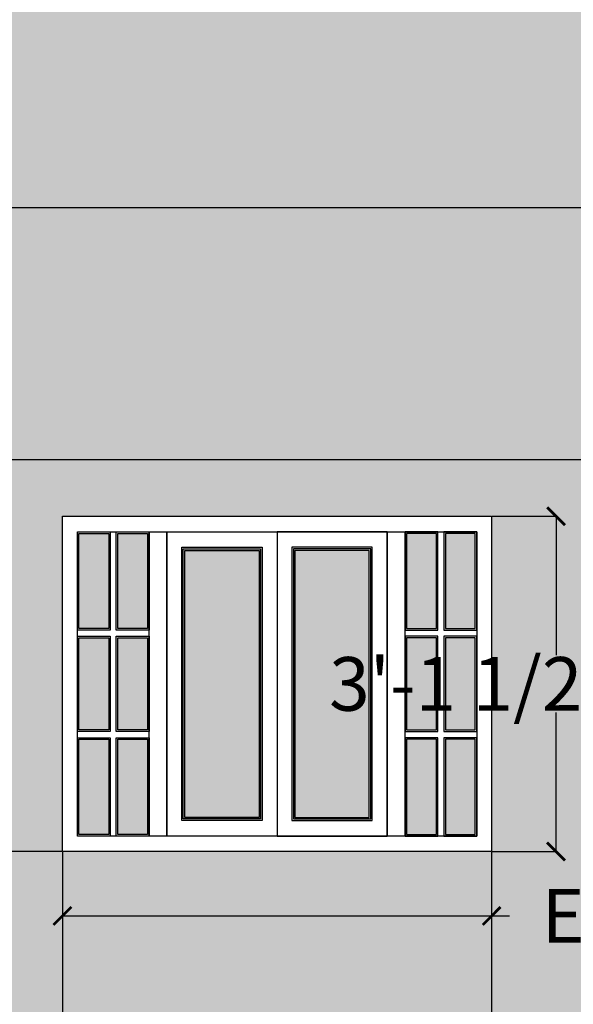
# Model space of a CAD drawing. Units: inches. Extents: x 528 to 2620, y -1066 to 798.
# Tile 37 of 41: x 2322 to 2384, y -1001 to -891. Entities that reach past the tile are written whole.
import ezdxf

# ---------------------------------------------------------------- set-up
doc = ezdxf.new("R2010")
doc.units = ezdxf.units.IN
doc.header["$MEASUREMENT"] = 0
for name, color, linetype, lineweight in [('A-ANNO-DIMS', 2, 'Continuous', 18), ('A-ELEV', 7, 'Continuous', 25), ('A-ELEV-PATT', 8, 'Continuous', 13)]:
    doc.layers.add(name, color=color, linetype=linetype, lineweight=lineweight)
doc.styles.get("Standard").update_dxf_attribs({"font": 'arial.ttf'})
doc.dimstyles.get("Standard").update_dxf_attribs({"dimtxt": 6, "dimasz": 2, "dimexe": 0.18, "dimexo": 0.0625, "dimgap": 0.09, "dimtad": 0, "dimtih": 1, "dimtoh": 1, "dimdec": 1, "dimzin": 0, "dimdsep": 46, "dimlunit": 3, "dimtxsty": 'Standard', "dimblk": 'ARCHTICK', "dimcen": 0.09, "dimadec": 0, "dimazin": 0, "dimtfac": 1, "dimtdec": 1, "dimtofl": 0, "dimtmove": 0, "dimatfit": 3, "dimfxl": 1, "dimtolj": 1, "dimtzin": 0, "dimarcsym": 0})

# ---------------------------------------------------------------- blocks, each defined once
blk = doc.blocks.new('ww')
at = {"color": 0, "linetype": 'ByBlock'}
for p, q in [((30.67, -16.13), (126.65, -16.13)), ((30.67, -91.08), (30.67, -16.13)), ((126.65, -16.13), (126.65, -91.08)), ((34.01, -19.6), (123.32, -19.6)), ((34.01, -87.61), (34.01, -19.6)), ((34.01, -19.6), (49.87, -19.6)), ((34.01, -87.61), (34.01, -19.6)), ((50.03, -87.61), (50.03, -19.6)), ((54.03, -19.6), (54.03, -87.61)), ((103.29, -19.6), (103.29, -87.61)), ((107.29, -87.61), (107.29, -19.6)), ((123.32, -19.6), (123.32, -87.61)), ((123.32, -87.61), (34.01, -87.61)), ((126.65, -91.08), (30.67, -91.08))]:
    blk.add_line(p, q, dxfattribs=at)
at = {"color": 0, "linetype": 'ByBlock', "ltscale": 25}
for p, q in [((34.01, -41.58), (34.01, -19.6)), ((34.01, -19.6), (41.35, -19.6)), ((41.35, -19.6), (41.35, -41.58)), ((42.69, -41.58), (42.69, -19.6)), ((42.69, -19.6), (50.03, -19.6)), ((50.03, -19.6), (50.03, -41.58)), ((54.03, -87.61), (54.03, -19.6)), ((54.03, -19.6), (78.66, -19.6)), ((103.29, -19.6), (78.66, -19.6)), ((78.66, -19.6), (78.66, -87.61)), ((78.66, -19.6), (78.66, -87.61)), ((103.29, -87.61), (103.29, -19.6)), ((107.29, -19.6), (107.29, -41.58)), ((114.63, -19.6), (107.29, -19.6)), ((114.63, -41.58), (114.63, -19.6)), ((115.97, -19.6), (115.97, -41.58)), ((123.32, -19.6), (115.97, -19.6)), ((123.32, -41.58), (123.32, -19.6)), ((34.34, -41.23), (34.34, -19.95)), ((34.34, -19.95), (41.02, -19.95)), ((41.02, -19.95), (41.02, -41.23)), ((43.02, -41.23), (43.02, -19.95)), ((43.02, -19.95), (49.7, -19.95)), ((49.7, -19.95), (49.7, -41.23)), ((107.62, -19.95), (107.62, -41.23)), ((114.3, -19.95), (107.62, -19.95)), ((114.3, -41.23), (114.3, -19.95)), ((116.3, -19.95), (116.3, -41.23)), ((122.98, -19.95), (116.3, -19.95)), ((122.98, -41.23), (122.98, -19.95)), ((57.37, -84.14), (57.37, -23.07)), ((57.37, -23.07), (75.33, -23.07)), ((57.7, -83.8), (57.7, -23.42)), ((57.7, -23.42), (74.99, -23.42)), ((58.03, -83.45), (58.03, -23.77)), ((58.03, -23.77), (74.66, -23.77)), ((74.66, -23.77), (74.66, -83.45)), ((74.99, -23.42), (74.99, -83.8)), ((75.33, -23.07), (75.33, -84.14)), ((99.96, -23.07), (81.99, -23.07)), ((81.99, -23.07), (81.99, -84.14)), ((99.62, -23.42), (82.33, -23.42)), ((82.33, -23.42), (82.33, -83.8)), ((99.29, -23.77), (82.66, -23.77)), ((82.66, -23.77), (82.66, -83.45)), ((99.29, -83.45), (99.29, -23.77)), ((99.62, -83.8), (99.62, -23.42)), ((99.96, -84.14), (99.96, -23.07)), ((41.35, -41.58), (34.01, -41.58)), ((41.02, -41.23), (34.34, -41.23)), ((50.03, -41.58), (42.69, -41.58)), ((49.7, -41.23), (43.02, -41.23)), ((107.29, -41.58), (114.63, -41.58)), ((107.62, -41.23), (114.3, -41.23)), ((115.97, -41.58), (123.32, -41.58)), ((116.3, -41.23), (122.98, -41.23)), ((34.01, -64.25), (34.01, -42.97)), ((34.01, -42.97), (41.35, -42.97)), ((34.34, -63.9), (34.34, -43.31)), ((34.34, -43.31), (41.02, -43.31)), ((41.02, -43.31), (41.02, -63.9)), ((41.35, -42.97), (41.35, -64.25)), ((42.69, -64.25), (42.69, -42.97)), ((42.69, -42.97), (50.03, -42.97)), ((43.02, -63.9), (43.02, -43.31)), ((43.02, -43.31), (49.7, -43.31)), ((49.7, -43.31), (49.7, -63.9)), ((50.03, -42.97), (50.03, -64.25)), ((107.29, -42.97), (107.29, -64.25)), ((114.63, -42.97), (107.29, -42.97)), ((107.62, -43.31), (107.62, -63.9)), ((114.3, -43.31), (107.62, -43.31)), ((114.3, -63.9), (114.3, -43.31)), ((114.63, -64.25), (114.63, -42.97)), ((115.97, -42.97), (115.97, -64.25)), ((123.32, -42.97), (115.97, -42.97)), ((116.3, -43.31), (116.3, -63.9)), ((122.98, -43.31), (116.3, -43.31)), ((122.98, -63.9), (122.98, -43.31)), ((123.32, -64.25), (123.32, -42.97)), ((41.35, -64.25), (34.01, -64.25)), ((34.01, -87.61), (34.01, -65.64)), ((34.01, -65.64), (41.35, -65.64)), ((41.02, -63.9), (34.34, -63.9)), ((34.34, -87.27), (34.34, -65.98)), ((34.34, -65.98), (41.02, -65.98)), ((41.02, -65.98), (41.02, -87.27)), ((41.35, -65.64), (41.35, -87.61)), ((50.03, -64.25), (42.69, -64.25)), ((42.69, -87.61), (42.69, -65.64)), ((42.69, -65.64), (50.03, -65.64)), ((49.7, -63.9), (43.02, -63.9)), ((43.02, -87.27), (43.02, -65.98)), ((43.02, -65.98), (49.7, -65.98)), ((49.7, -65.98), (49.7, -87.27)), ((50.03, -65.64), (50.03, -87.61)), ((107.29, -64.25), (114.63, -64.25)), ((107.29, -65.64), (107.29, -87.61)), ((114.63, -65.64), (107.29, -65.64)), ((107.62, -63.9), (114.3, -63.9)), ((107.62, -65.98), (107.62, -87.27)), ((114.3, -65.98), (107.62, -65.98)), ((114.3, -87.27), (114.3, -65.98)), ((114.63, -87.61), (114.63, -65.64)), ((115.97, -64.25), (123.32, -64.25)), ((115.97, -65.64), (115.97, -87.61)), ((123.32, -65.64), (115.97, -65.64)), ((116.3, -63.9), (122.98, -63.9)), ((116.3, -65.98), (116.3, -87.27)), ((122.98, -65.98), (116.3, -65.98)), ((122.98, -87.27), (122.98, -65.98)), ((123.32, -87.61), (123.32, -65.64)), ((74.66, -83.45), (58.03, -83.45)), ((82.66, -83.45), (99.29, -83.45)), ((75.33, -84.14), (57.37, -84.14)), ((74.99, -83.8), (57.7, -83.8)), ((81.99, -84.14), (99.96, -84.14)), ((82.33, -83.8), (99.62, -83.8)), ((41.35, -87.61), (34.01, -87.61)), ((41.02, -87.27), (34.34, -87.27)), ((50.03, -87.61), (42.69, -87.61)), ((49.7, -87.27), (43.02, -87.27)), ((78.66, -87.61), (54.03, -87.61)), ((78.66, -87.61), (103.29, -87.61)), ((107.29, -87.61), (114.63, -87.61)), ((107.62, -87.27), (114.3, -87.27)), ((115.97, -87.61), (123.32, -87.61)), ((116.3, -87.27), (122.98, -87.27))]:
    blk.add_line(p, q, dxfattribs=at)
blk = doc.blocks.new('_ArchTick')
at = {"color": 0, "linetype": 'ByBlock', "const_width": 0.15}
blk.add_lwpolyline([(-0.5, -0.5), (0.5, 0.5)], dxfattribs=at)
blk = doc.blocks.new('*D54')
at = {"layer": 'A-ANNO-DIMS', "color": 0, "lineweight": -2, "transparency": 16777216}
for p, q in [((2327.05, -984.21), (2327.05, -991.53)), ((2375.05, -984.21), (2375.05, -991.53)), ((2327.05, -991.35), (2375.05, -991.35)), ((2375.05, -991.35), (2377.05, -991.35))]:
    blk.add_line(p, q, dxfattribs=at)
at = {"layer": 'Defpoints', "color": 0, "transparency": 16777216}
for p in [(2327.05, -984.15), (2375.05, -984.15), (2375.05, -991.35)]:
    blk.add_point(p, dxfattribs=at)
at = {"layer": 'A-ANNO-DIMS', "color": 0, "lineweight": -2, "transparency": 16777216, "xscale": 2, "yscale": 2, "zscale": 2, "rotation": 180}
blk.add_blockref('_ArchTick', (2327.05, -991.35), dxfattribs=at)
at = {"layer": 'A-ANNO-DIMS', "color": 0, "lineweight": -2, "transparency": 16777216, "xscale": 2, "yscale": 2, "zscale": 2}
blk.add_blockref('_ArchTick', (2375.05, -991.35), dxfattribs=at)
at = {"layer": 'A-ANNO-DIMS', "color": 0, "transparency": 16777216, "insert": (2439.5, -991.35), "char_height": 6, "attachment_point": 5}
blk.add_mtext('\\A1;ELEVATION WINDOW 4\'-0" TYP.', dxfattribs=at)
blk = doc.blocks.new('*D55')
at = {"layer": 'A-ANNO-DIMS', "color": 0, "lineweight": -2, "transparency": 16777216}
for p, q in [((2375.11, -946.66), (2382.43, -946.66)), ((2382.25, -946.66), (2382.25, -962.21)), ((2382.25, -984.15), (2382.25, -968.6)), ((2375.11, -984.15), (2382.43, -984.15))]:
    blk.add_line(p, q, dxfattribs=at)
at = {"layer": 'Defpoints', "color": 0, "transparency": 16777216}
for p in [(2375.05, -946.66), (2382.25, -946.66), (2375.05, -984.15)]:
    blk.add_point(p, dxfattribs=at)
at = {"layer": 'A-ANNO-DIMS', "color": 0, "lineweight": -2, "transparency": 16777216, "xscale": 2, "yscale": 2, "zscale": 2}
for p, rotation in [((2382.25, -946.66), 90), ((2382.25, -984.15), 270)]:
    blk.add_blockref('_ArchTick', p, dxfattribs=dict(at, rotation=rotation))
at = {"layer": 'A-ANNO-DIMS', "color": 0, "transparency": 16777216, "insert": (2382.25, -965.41), "char_height": 6, "attachment_point": 5}
blk.add_mtext('\\A1;3\'-1 1/2" TYP.', dxfattribs=at)
blk = doc.blocks.new('*D71')
at = {"layer": 'A-ANNO-DIMS', "color": 0, "lineweight": -2, "transparency": 16777216}
for p, q in [((2326.98, -984.15), (2243.87, -984.15)), ((2244.05, -984.15), (2244.05, -998.99)), ((2244.05, -1020.15), (2244.05, -1005.3)), ((2298.48, -1020.15), (2243.87, -1020.15))]:
    blk.add_line(p, q, dxfattribs=at)
at = {"layer": 'Defpoints', "color": 0, "transparency": 16777216}
for p in [(2244.05, -984.15), (2327.05, -984.15), (2298.55, -1020.15)]:
    blk.add_point(p, dxfattribs=at)
at = {"layer": 'A-ANNO-DIMS', "color": 0, "lineweight": -2, "transparency": 16777216, "xscale": 2, "yscale": 2, "zscale": 2}
for p, rotation in [((2244.05, -984.15), 90), ((2244.05, -1020.15), 270)]:
    blk.add_blockref('_ArchTick', p, dxfattribs=dict(at, rotation=rotation))
at = {"layer": 'A-ANNO-DIMS', "color": 0, "transparency": 16777216, "insert": (2244.05, -1002.15), "char_height": 6, "attachment_point": 5}
blk.add_mtext('\\A1;3\'-0"', dxfattribs=at)
blk = doc.blocks.new('*D72')
at = {"layer": 'A-ANNO-DIMS', "color": 0, "lineweight": -2, "transparency": 16777216}
for p, q in [((2394.48, -940.36), (2243.87, -940.36)), ((2244.05, -940.36), (2244.05, -959.1)), ((2244.05, -984.15), (2244.05, -965.41)), ((2326.98, -984.15), (2243.87, -984.15))]:
    blk.add_line(p, q, dxfattribs=at)
at = {"layer": 'Defpoints', "color": 0, "transparency": 16777216}
for p in [(2244.05, -940.36), (2394.55, -940.36), (2327.05, -984.15)]:
    blk.add_point(p, dxfattribs=at)
at = {"layer": 'A-ANNO-DIMS', "color": 0, "lineweight": -2, "transparency": 16777216, "xscale": 2, "yscale": 2, "zscale": 2}
for p, rotation in [((2244.05, -940.36), 90), ((2244.05, -984.15), 270)]:
    blk.add_blockref('_ArchTick', p, dxfattribs=dict(at, rotation=rotation))
at = {"layer": 'A-ANNO-DIMS', "color": 0, "transparency": 16777216, "insert": (2244.05, -962.26), "char_height": 6, "attachment_point": 5}
blk.add_mtext('\\A1;3\'-8"', dxfattribs=at)
blk = doc.blocks.new('*D73')
at = {"layer": 'A-ANNO-DIMS', "color": 0, "lineweight": -2, "transparency": 16777216}
for p, q in [((2265.98, -912.15), (2243.87, -912.15)), ((2244.05, -912.15), (2244.05, -923.15)), ((2244.05, -940.36), (2244.05, -929.36)), ((2394.48, -940.36), (2243.87, -940.36))]:
    blk.add_line(p, q, dxfattribs=at)
at = {"layer": 'Defpoints', "color": 0, "transparency": 16777216}
for p in [(2244.05, -912.15), (2266.05, -912.15), (2394.55, -940.36)]:
    blk.add_point(p, dxfattribs=at)
at = {"layer": 'A-ANNO-DIMS', "color": 0, "lineweight": -2, "transparency": 16777216, "xscale": 2, "yscale": 2, "zscale": 2}
for p, rotation in [((2244.05, -912.15), 90), ((2244.05, -940.36), 270)]:
    blk.add_blockref('_ArchTick', p, dxfattribs=dict(at, rotation=rotation))
at = {"layer": 'A-ANNO-DIMS', "color": 0, "transparency": 16777216, "insert": (2244.05, -926.26), "char_height": 6, "attachment_point": 5}
blk.add_mtext('\\A1;2\'-4"', dxfattribs=at)
blk = doc.blocks.new('*D81')
at = {"layer": 'A-ANNO-DIMS', "color": 0, "lineweight": -2, "transparency": 16777216}
for p, q in [((2327.05, -984.21), (2327.05, -1042.33)), ((2298.55, -1020.21), (2298.55, -1042.33)), ((2298.55, -1042.15), (2327.05, -1042.15)), ((2327.05, -1042.15), (2329.05, -1042.15))]:
    blk.add_line(p, q, dxfattribs=at)
at = {"layer": 'Defpoints', "color": 0, "transparency": 16777216}
for p in [(2327.05, -984.15), (2298.55, -1020.15), (2327.05, -1042.15)]:
    blk.add_point(p, dxfattribs=at)
at = {"layer": 'A-ANNO-DIMS', "color": 0, "lineweight": -2, "transparency": 16777216, "xscale": 2, "yscale": 2, "zscale": 2, "rotation": 180}
blk.add_blockref('_ArchTick', (2298.55, -1042.15), dxfattribs=at)
at = {"layer": 'A-ANNO-DIMS', "color": 0, "lineweight": -2, "transparency": 16777216, "xscale": 2, "yscale": 2, "zscale": 2}
blk.add_blockref('_ArchTick', (2327.05, -1042.15), dxfattribs=at)
at = {"layer": 'A-ANNO-DIMS', "color": 0, "transparency": 16777216, "insert": (2344.15, -1042.15), "char_height": 6, "attachment_point": 5}
blk.add_mtext('\\A1;2\'-4 1/2"', dxfattribs=at)
blk = doc.blocks.new('*D82')
at = {"layer": 'A-ANNO-DIMS', "color": 0, "lineweight": -2, "transparency": 16777216}
for p, q in [((2327.05, -984.21), (2327.05, -1042.33)), ((2375.05, -984.21), (2375.05, -1042.33)), ((2327.05, -1042.15), (2342.86, -1042.15)), ((2375.05, -1042.15), (2359.23, -1042.15))]:
    blk.add_line(p, q, dxfattribs=at)
at = {"layer": 'Defpoints', "color": 0, "transparency": 16777216}
for p in [(2327.05, -984.15), (2375.05, -984.15), (2375.05, -1042.15)]:
    blk.add_point(p, dxfattribs=at)
at = {"layer": 'A-ANNO-DIMS', "color": 0, "lineweight": -2, "transparency": 16777216, "xscale": 2, "yscale": 2, "zscale": 2, "rotation": 180}
blk.add_blockref('_ArchTick', (2327.05, -1042.15), dxfattribs=at)
at = {"layer": 'A-ANNO-DIMS', "color": 0, "lineweight": -2, "transparency": 16777216, "xscale": 2, "yscale": 2, "zscale": 2}
blk.add_blockref('_ArchTick', (2375.05, -1042.15), dxfattribs=at)
at = {"layer": 'A-ANNO-DIMS', "color": 0, "transparency": 16777216, "insert": (2351.05, -1042.15), "char_height": 6, "attachment_point": 5}
blk.add_mtext('\\A1;4\'-0"', dxfattribs=at)
blk = doc.blocks.new('*D83')
at = {"layer": 'A-ANNO-DIMS', "color": 0, "lineweight": -2, "transparency": 16777216}
for p, q in [((2375.05, -984.21), (2375.05, -1042.33)), ((2394.55, -1020.21), (2394.55, -1042.33)), ((2375.05, -1042.15), (2394.55, -1042.15)), ((2394.55, -1042.15), (2396.55, -1042.15))]:
    blk.add_line(p, q, dxfattribs=at)
at = {"layer": 'Defpoints', "color": 0, "transparency": 16777216}
for p in [(2375.05, -984.15), (2394.55, -1020.15), (2394.55, -1042.15)]:
    blk.add_point(p, dxfattribs=at)
at = {"layer": 'A-ANNO-DIMS', "color": 0, "lineweight": -2, "transparency": 16777216, "xscale": 2, "yscale": 2, "zscale": 2, "rotation": 180}
blk.add_blockref('_ArchTick', (2375.05, -1042.15), dxfattribs=at)
at = {"layer": 'A-ANNO-DIMS', "color": 0, "lineweight": -2, "transparency": 16777216, "xscale": 2, "yscale": 2, "zscale": 2}
blk.add_blockref('_ArchTick', (2394.55, -1042.15), dxfattribs=at)
at = {"layer": 'A-ANNO-DIMS', "color": 0, "transparency": 16777216, "insert": (2411.32, -1042.15), "char_height": 6, "attachment_point": 5}
blk.add_mtext('\\A1;1\'-7 1/2"', dxfattribs=at)

msp = doc.modelspace()

# ---------------------------------------------------------------- hatches: boundary and pattern name
at = {"layer": 'A-ELEV-PATT', "transparency": 33554687}
h = msp.add_hatch(color=256, dxfattribs=at)
h.dxf.hatch_style = 1
h.paths.add_polyline_path([(2448.55, -756.15), (2270.55, -756.15), (2270.55, -780.15), (2436.55, -780.15), (2436.55, -888.15), (2266.05, -888.15), (2266.05, -912.15), (2448.55, -912.15)])
h = msp.add_hatch(color=256, dxfattribs=at)
h.dxf.hatch_style = 1
h.paths.add_polyline_path([(2586.55, -912.15), (2448.55, -912.15), (2448.55, -940.66), (2547.55, -940.66), (2547.55, -990.15), (2448.55, -990.15), (2448.55, -1020.15), (2586.55, -1020.15)])
h.paths.add_polyline_path([(2481.55, -789.84), (2562.55, -789.84), (2562.55, -761.55), (2448.55, -761.55), (2448.55, -900.15), (2562.55, -900.15), (2562.55, -876.97), (2481.55, -876.97), (2481.55, -833.41)])
h.paths.add_polyline_path([(2412.55, -780.15), (2298.55, -780.15), (2298.55, -852.15), (2322.55, -852.15), (2322.55, -814.66), (2370.55, -814.66), (2370.55, -852.15), (2412.55, -852.15)])
h.paths.add_polyline_path([(2394.55, -940.36), (2442.55, -940.36), (2442.55, -1020.15), (2448.55, -1020.15), (2448.55, -990.15), (2448.55, -912.15), (2310.55, -912.15), (2310.55, -1020.15), (2394.55, -1020.15)])
h.paths.add_polyline_path([(2327.05, -984.15), (2327.05, -946.66), (2375.05, -946.66), (2375.05, -984.15)], flags=16)
h.paths.add_polyline_path([(2328.71, -982.41), (2328.71, -948.4), (2336.65, -948.4), (2336.73, -948.4), (2373.38, -948.4), (2373.38, -982.41), (2369.7, -982.41)], flags=0)
h.paths.add_polyline_path([(2338.73, -982.41), (2338.73, -948.4), (2351.05, -948.4), (2363.36, -948.4), (2363.36, -982.41), (2351.05, -982.41)], flags=0)
h.paths.add_polyline_path([(2340.4, -980.68), (2340.4, -950.13), (2349.38, -950.13), (2349.38, -980.68)], flags=0)
h.paths.add_polyline_path([(2340.73, -980.33), (2340.73, -950.48), (2349.05, -950.48), (2349.05, -980.33)], flags=0)
h.paths.add_polyline_path([(2352.71, -980.68), (2352.71, -950.13), (2361.7, -950.13), (2361.7, -980.68)], flags=0)
h.paths.add_polyline_path([(2353.05, -980.33), (2353.05, -950.48), (2361.36, -950.48), (2361.36, -980.33)], flags=0)
h.paths.add_polyline_path([(2336.73, -982.41), (2333.05, -982.41), (2333.05, -971.42), (2336.73, -971.42), (2336.73, -970.73), (2333.05, -970.73), (2333.05, -960.08), (2336.73, -960.08), (2336.73, -959.39), (2333.05, -959.39), (2333.05, -948.57), (2336.73, -948.57)], flags=0)
h.paths.add_polyline_path([(2333.22, -982.24), (2333.22, -971.6), (2336.73, -971.6), (2336.73, -982.24)], flags=0)
h.paths.add_polyline_path([(2332.39, -982.41), (2328.71, -982.41), (2328.71, -948.4), (2332.39, -948.4), (2332.39, -959.39), (2328.71, -959.39), (2328.71, -960.08), (2332.39, -960.08), (2332.39, -970.73), (2328.71, -970.73), (2328.71, -971.42), (2332.39, -971.42)], flags=0)
h.paths.add_polyline_path([(2332.22, -982.24), (2328.71, -982.24), (2328.71, -971.6), (2332.22, -971.6)], flags=0)
h.paths.add_polyline_path([(2365.36, -982.41), (2365.36, -948.4), (2369.04, -948.4), (2369.04, -959.39), (2365.36, -959.39), (2365.36, -960.08), (2369.04, -960.08), (2369.04, -970.73), (2365.36, -970.73), (2365.36, -971.42), (2369.04, -971.42), (2369.04, -982.41)], flags=0)
h.paths.add_polyline_path([(2369.7, -971.42), (2373.38, -971.42), (2373.38, -982.24), (2369.7, -982.24)], flags=0)
h.paths.add_polyline_path([(2333.22, -970.55), (2333.22, -960.26), (2336.73, -960.26), (2336.73, -970.55)], flags=0)
h.paths.add_polyline_path([(2332.22, -970.55), (2328.71, -970.55), (2328.71, -960.26), (2332.22, -960.26)], flags=0)
h.paths.add_polyline_path([(2369.7, -970.73), (2369.7, -960.08), (2373.38, -960.08), (2373.38, -970.73)], flags=0)
h.paths.add_polyline_path([(2336.56, -959.22), (2336.56, -948.57), (2336.73, -948.4), (2336.73, -959.22)], flags=0)
h.paths.add_polyline_path([(2332.22, -959.22), (2328.71, -959.22), (2328.71, -948.57), (2332.22, -948.57)], flags=0)
h.paths.add_polyline_path([(2369.7, -959.39), (2369.7, -948.4), (2373.38, -948.4), (2373.38, -959.39)], flags=0)
h = msp.add_hatch(color=256, dxfattribs=at)
h.dxf.hatch_style = 1
h.paths.add_polyline_path([(2527.86, -818.48), (2519.55, -818.48), (2519.55, -848.33), (2527.86, -848.33)])
h.paths.add_polyline_path([(2515.55, -818.48), (2507.23, -818.48), (2507.23, -848.33), (2515.55, -848.33)])
h.paths.add_polyline_path([(2498.72, -816.57), (2495.38, -816.57), (2495.38, -827.22), (2498.72, -827.22)])
h.paths.add_polyline_path([(2503.06, -816.57), (2499.72, -816.57), (2499.72, -827.22), (2503.06, -827.22)])
h.paths.add_polyline_path([(2498.72, -828.26), (2495.38, -828.26), (2495.38, -838.55), (2498.72, -838.55)])
h.paths.add_polyline_path([(2503.06, -828.26), (2499.72, -828.26), (2499.72, -838.55), (2503.06, -838.55)])
h.paths.add_polyline_path([(2498.72, -839.6), (2495.38, -839.6), (2495.38, -850.24), (2498.72, -850.24)])
h.paths.add_polyline_path([(2503.06, -839.6), (2499.72, -839.6), (2499.72, -850.24), (2503.06, -850.24)])
h.paths.add_polyline_path([(2535.37, -839.6), (2532.03, -839.6), (2532.03, -850.24), (2535.37, -850.24)])
h.paths.add_polyline_path([(2539.71, -839.6), (2536.37, -839.6), (2536.37, -850.24), (2539.71, -850.24)])
h.paths.add_polyline_path([(2535.37, -828.26), (2532.03, -828.26), (2532.03, -838.55), (2535.37, -838.55)])
h.paths.add_polyline_path([(2539.71, -828.26), (2536.37, -828.26), (2536.37, -838.55), (2539.71, -838.55)])
h.paths.add_polyline_path([(2535.37, -816.57), (2532.03, -816.57), (2532.03, -827.22), (2535.37, -827.22)])
h.paths.add_polyline_path([(2356.86, -818.48), (2348.55, -818.48), (2348.55, -848.33), (2356.86, -848.33)])
h.paths.add_polyline_path([(2344.55, -818.48), (2336.23, -818.48), (2336.23, -848.33), (2344.55, -848.33)])
h.paths.add_polyline_path([(2327.72, -816.57), (2324.38, -816.57), (2324.38, -827.22), (2327.72, -827.22)])
h.paths.add_polyline_path([(2332.06, -816.57), (2328.72, -816.57), (2328.72, -827.22), (2332.06, -827.22)])
h.paths.add_polyline_path([(2327.72, -828.26), (2324.38, -828.26), (2324.38, -838.55), (2327.72, -838.55)])
h.paths.add_polyline_path([(2332.06, -828.26), (2328.72, -828.26), (2328.72, -838.55), (2332.06, -838.55)])
h.paths.add_polyline_path([(2327.72, -839.6), (2324.38, -839.6), (2324.38, -850.24), (2327.72, -850.24)])
h.paths.add_polyline_path([(2332.06, -839.6), (2328.72, -839.6), (2328.72, -850.24), (2332.06, -850.24)])
h.paths.add_polyline_path([(2368.71, -839.6), (2365.37, -839.6), (2365.37, -850.24), (2368.71, -850.24)])
h.paths.add_polyline_path([(2364.37, -839.6), (2361.03, -839.6), (2361.03, -850.24), (2364.37, -850.24)])
h.paths.add_polyline_path([(2364.37, -828.26), (2361.03, -828.26), (2361.03, -838.55), (2364.37, -838.55)])
h.paths.add_polyline_path([(2368.71, -828.26), (2365.37, -828.26), (2365.37, -838.55), (2368.71, -838.55)])
h.paths.add_polyline_path([(2364.37, -816.57), (2361.03, -816.57), (2361.03, -827.22), (2364.37, -827.22)])
h.paths.add_polyline_path([(2368.71, -816.57), (2365.37, -816.57), (2365.37, -827.22), (2368.71, -827.22)])
h.paths.add_polyline_path([(2361.36, -950.48), (2353.05, -950.48), (2353.05, -980.33), (2361.36, -980.33)])
h.paths.add_polyline_path([(2349.05, -950.48), (2340.73, -950.48), (2340.73, -980.33), (2349.05, -980.33)])
h.paths.add_polyline_path([(2336.56, -971.6), (2333.22, -971.6), (2333.22, -982.24), (2336.56, -982.24)])
h.paths.add_polyline_path([(2332.22, -971.6), (2328.88, -971.6), (2328.88, -982.24), (2332.22, -982.24)])
h.paths.add_polyline_path([(2336.56, -960.26), (2333.22, -960.26), (2333.22, -970.55), (2336.56, -970.55)])
h.paths.add_polyline_path([(2332.22, -960.26), (2328.88, -960.26), (2328.88, -970.55), (2332.22, -970.55)])
h.paths.add_polyline_path([(2332.22, -948.57), (2328.88, -948.57), (2328.88, -959.22), (2332.22, -959.22)])
h.paths.add_polyline_path([(2336.56, -948.57), (2333.22, -948.57), (2333.22, -959.22), (2336.56, -959.22)])
h.paths.add_polyline_path([(2368.87, -971.6), (2365.53, -971.6), (2365.53, -982.24), (2368.87, -982.24)])
h.paths.add_polyline_path([(2373.21, -971.6), (2369.87, -971.6), (2369.87, -982.24), (2373.21, -982.24)])
h.paths.add_polyline_path([(2373.21, -960.26), (2369.87, -960.26), (2369.87, -970.55), (2373.21, -970.55)])
h.paths.add_polyline_path([(2368.87, -960.26), (2365.53, -960.26), (2365.53, -970.55), (2368.87, -970.55)])
h.paths.add_polyline_path([(2368.87, -948.57), (2365.53, -948.57), (2365.53, -959.22), (2368.87, -959.22)])
h.paths.add_polyline_path([(2373.21, -948.57), (2369.87, -948.57), (2369.87, -959.22), (2373.21, -959.22)])
h.paths.add_polyline_path([(2527.86, -950.48), (2519.55, -950.48), (2519.55, -980.33), (2527.86, -980.33)])
h.paths.add_polyline_path([(2515.55, -950.48), (2507.23, -950.48), (2507.23, -980.33), (2515.55, -980.33)])
h.paths.add_polyline_path([(2539.71, -971.6), (2536.37, -971.6), (2536.37, -982.24), (2539.71, -982.24)])
h.paths.add_polyline_path([(2535.37, -971.6), (2532.03, -971.6), (2532.03, -982.24), (2535.37, -982.24)])
h.paths.add_polyline_path([(2535.37, -960.26), (2532.03, -960.26), (2532.03, -970.55), (2535.37, -970.55)])
h.paths.add_polyline_path([(2539.71, -960.26), (2536.37, -960.26), (2536.37, -970.55), (2539.71, -970.55)])
h.paths.add_polyline_path([(2535.37, -948.57), (2532.03, -948.57), (2532.03, -959.22), (2535.37, -959.22)])
h.paths.add_polyline_path([(2539.71, -948.57), (2536.37, -948.57), (2536.37, -959.22), (2539.71, -959.22)])
h.paths.add_polyline_path([(2498.72, -971.6), (2495.38, -971.6), (2495.38, -982.24), (2498.72, -982.24)])
h.paths.add_polyline_path([(2503.06, -971.6), (2499.72, -971.6), (2499.72, -982.24), (2503.06, -982.24)])
h.paths.add_polyline_path([(2498.72, -960.26), (2495.38, -960.26), (2495.38, -970.55), (2498.72, -970.55)])
h.paths.add_polyline_path([(2503.06, -960.26), (2499.72, -960.26), (2499.72, -970.55), (2503.06, -970.55)])
h.paths.add_polyline_path([(2498.72, -948.57), (2495.38, -948.57), (2495.38, -959.22), (2498.72, -959.22)])
h.paths.add_polyline_path([(2503.06, -948.57), (2499.72, -948.57), (2499.72, -959.22), (2503.06, -959.22)])

# ---------------------------------------------------------------- linework, layer by layer
at = {"layer": 'A-ELEV'}
msp.add_line((2266.05, -912.15), (2448.55, -912.15), dxfattribs=at)

# ---------------------------------------------------------------- block references
at = {"layer": 'A-ELEV', "xscale": 0.5001250312578946, "yscale": 0.5001250312578946, "zscale": 0.5001250312578946}
msp.add_blockref('ww', (2311.71, -938.6), dxfattribs=at)

# ---------------------------------------------------------------- dimensions: what is measured, and where the dimension line sits
at = {"layer": 'A-ANNO-DIMS'}
for base, p1, p2, picture, middle in [((2244.05, -912.15), (2394.55, -940.36), (2266.05, -912.15), '*D73', (2244.05, -926.26)), ((2244.05, -940.36), (2327.05, -984.15), (2394.55, -940.36), '*D72', (2244.05, -962.26)), ((2244.05, -984.15), (2298.55, -1020.15), (2327.05, -984.15), '*D71', (2244.05, -1002.15))]:
    dim = msp.add_linear_dim(base=base, p1=p1, p2=p2, angle=90, dimstyle='Standard', override={"dimdec": 1, "dimlfac": 1, "dimrnd": 0, "dimzin": 1, "dimdsep": 46, "dimlunit": 4, "dimfrac": 2}, dxfattribs=at)
    dim.commit()
    dim.dimension.update_dxf_attribs({"geometry": picture, "text_midpoint": middle})
dim = msp.add_linear_dim(base=(2382.25, -946.66), p1=(2375.05, -984.15), p2=(2375.05, -946.66), angle=90, text='<> TYP.', dimstyle='Standard', override={"dimdec": 1, "dimrnd": 0, "dimzin": 1, "dimlunit": 4, "dimfrac": 2}, dxfattribs=at)
dim.commit()
dim.dimension.update_dxf_attribs({"geometry": '*D55', "text_midpoint": (2382.25, -965.41)})
dim = msp.add_linear_dim(base=(2375.05, -991.35), p1=(2327.05, -984.15), p2=(2375.05, -984.15), text='ELEVATION WINDOW <> TYP.', dimstyle='Standard', override={"dimdec": 1, "dimrnd": 0, "dimzin": 1, "dimlunit": 4, "dimfrac": 2}, dxfattribs=at)
dim.commit()
dim.dimension.update_dxf_attribs({"geometry": '*D54', "text_midpoint": (2439.5, -991.35)})
for base, p1, p2, picture, middle in [((2327.05, -1042.15), (2298.55, -1020.15), (2327.05, -984.15), '*D81', (2344.15, -1042.15)), ((2375.05, -1042.15), (2327.05, -984.15), (2375.05, -984.15), '*D82', (2351.05, -1042.15)), ((2394.55, -1042.15), (2375.05, -984.15), (2394.55, -1020.15), '*D83', (2411.32, -1042.15))]:
    dim = msp.add_linear_dim(base=base, p1=p1, p2=p2, dimstyle='Standard', override={"dimdec": 1, "dimlfac": 1, "dimrnd": 0, "dimzin": 1, "dimdsep": 46, "dimlunit": 4, "dimfrac": 2}, dxfattribs=at)
    dim.commit()
    dim.dimension.update_dxf_attribs({"geometry": picture, "text_midpoint": middle})

doc.saveas('drawing.dxf')
